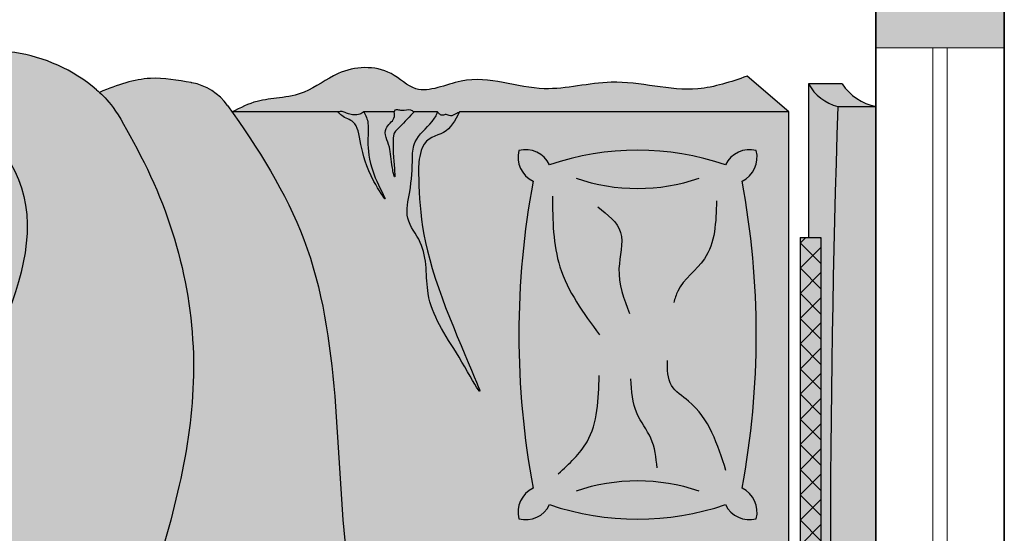
# Model space of a CAD drawing. Units: inches. Extents: x 3148 to 3962, y 1142 to 1671.
# Tile 5 of 9: x 3413 to 3482, y 1483 to 1519. Entities that reach past the tile are written whole.
import ezdxf

# ---------------------------------------------------------------- set-up
doc = ezdxf.new("R2010")
doc.units = ezdxf.units.IN
for name, color, linetype, lineweight in [('A-FURN', 8, 'Continuous', 18), ('A-GLAZ', 4, 'Continuous', 18), ('A-WALL', 7, 'Continuous', 35), ('estofado', 7, 'Continuous', 25)]:
    doc.layers.add(name, color=color, linetype=linetype, lineweight=lineweight)
doc.layers.add('A-WALL-PATT', color=252, linetype='Continuous', lineweight=13, true_color=0x939598)

# ---------------------------------------------------------------- blocks, each defined once
blk = doc.blocks.new('Cama Box Regencia LOLA')
at = {"layer": 'estofado', "ltscale": 0.2}
h = blk.add_hatch(color=256, dxfattribs=at)
h.dxf.hatch_style = 1
h.set_gradient(color1=(139, 102, 75), color2=(43, 31, 23), one_color=1, tint=0.1299999952316284)
h.paths.add_polyline_path([(-0.8097611300671587, -0.0676434826297623), (-0.8097611300671587, 0, -0.1973270565007711), (-0.8500000000000227, -0.060000000000116), (-0.8500000000000227, -0.1200000000000045, 0.2083477308151313)])
h = blk.add_hatch(color=256, dxfattribs=at)
h.dxf.hatch_style = 1
h.set_gradient(color1=(139, 102, 75), color2=(43, 31, 23), one_color=1, tint=0.1299999952316284, name='CURVED')
h.paths.add_polyline_path([(0.8097611300672723, 0), (-0.8097611300671587, 0), (-0.8097611300671587, -0.0676434826297054, 0.0166383680674931), (0.8097611300672723, -0.0676434823212162)])
h = blk.add_hatch(color=256, dxfattribs=at)
h.dxf.hatch_style = 1
h.set_gradient(color1=(139, 102, 75), color2=(43, 31, 23), one_color=1, tint=0.1299999952316284, name='INVCURVED')
h.paths.add_polyline_path([(0.8097611299908749, -0.0676434823237742, -0.0166383680667078), (-0.8097611300671587, -0.0676434826297623, -0.2083477308153697), (-0.8500000000001364, -0.1200000000000045), (-0.5763381074484643, -0.1200000000000045), (-0.5763381074485779, -0.0977075818103117), (0.5763381073808205, -0.0977075818103117), (0.5763381073808205, -0.1200000000000045), (0.8500000000000227, -0.1200000000000045, -0.2083477318100794)])
h = blk.add_hatch(color=256, dxfattribs=at)
h.dxf.hatch_style = 1
h.set_gradient(color1=(139, 102, 75), color2=(198, 169, 149), one_color=1, tint=0.6800000071525574, name='CYLINDER')
h.paths.add_polyline_path([(0.5763381073808205, -0.0977075818103686), (-0.5763381074484643, -0.0977075818103117), (-0.5763381074485779, -0.1348263709859339), (0.5763381073808205, -0.134826370985877)])
h = blk.add_hatch(dxfattribs=at)
h.set_pattern_fill('ANSI37,_O', color=256, scale=0.01)
h.set_pattern_definition([(45, (-24.74368160026529, -44.17612681992631), (-0.0224506403026729, 0.0224506403026729), []), (135, (-24.74368160026529, -44.17612681992631), (-0.0224506403026729, -0.0224506403026729), [])])
h.paths.add_polyline_path([(0.5763381073808205, -0.0977075818103686), (-0.5763381074484643, -0.0977075818103117), (-0.5763381074485779, -0.1348263709859339), (0.5763381073808205, -0.134826370985877)])
h = blk.add_hatch(color=256, dxfattribs=at)
h.dxf.hatch_style = 1
h.set_gradient(color1=(240, 232, 219), color2=(213, 190, 154), one_color=1, tint=0.7200000286102295)
edge = h.paths.add_edge_path()
edge.add_line((-0.8000000000000682, -0.1548023628405417), (-0.863597199697665, -0.2293271111754507))
edge.add_spline(control_points=[(-0.8635971996977787, -0.2293271111754507), (-0.8537222782123308, -0.258285373872468), (-0.8269013755602826, -0.3369378214810581), (-0.8674912876567759, -0.4595932758330151), (-0.8253488717912205, -0.6001498518888299), (-0.8771423076391329, -0.7139760714239288), (-0.8243323781925938, -0.8129899320257435), (-0.885044987287756, -0.8716602542656914), (-0.879518062107536, -0.9542863467743244), (-0.8339551707063037, -1.008464155856984), (-0.8245672924600739, -1.059984630119799), (-0.8208601923470268, -1.104655887174089), (-0.8073908324747662, -1.131238421004809), (-0.7999999999999546, -1.145824641594799)], knot_values=[0, 0, 0, 0, 0.0901802310564388, 0.2449351320798513, 0.3646438241986237, 0.5132330690395209, 0.5950634960661151, 0.646820388242338, 0.740988272125753, 0.8098674202588053, 0.8551784313864677, 0.8950360916221496, 0.9434986994854018, 0.9434986994854018, 0.9434986994854018, 0.9434986994854018], degree=3, periodic=0)
edge.add_line((-0.7999999999999546, -1.145824641594856), (-0.7999999999999546, -0.9571831923306604))
edge.add_spline(control_points=[(-0.8000000000001818, -0.9571831923294098), (-0.8003674620557603, -0.9560020588672273), (-0.8014778173377408, -0.9524330433489467), (-0.799534669348418, -0.9460450666617248), (-0.7963405736333016, -0.9382358308520792), (-0.7944188048602429, -0.9289040147384638), (-0.7953122817383474, -0.9190683391483389), (-0.7985341887020923, -0.9137677522519994), (-0.7999999999999546, -0.911356242470788)], knot_values=[0, 0, 0, 0, 0.0036609130031785, 0.0110621328900358, 0.0190316076023675, 0.0292873612819121, 0.0393286152452009, 0.0477100398955968, 0.0477100398955968, 0.0477100398955968, 0.0477100398955968], degree=3, periodic=0)
edge.add_line((-0.8000000000000682, -0.9113562424705037), (-0.7999999999999546, -0.8573491405791173))
edge.add_spline(control_points=[(-0.7999999999999546, -0.8573491405791173), (-0.8011509914009592, -0.8570771933481751), (-0.804102924754261, -0.8563797336621519), (-0.8039036519178353, -0.8498286502876908), (-0.8010279369466388, -0.8413595542568258), (-0.805623441450507, -0.8302818657685406), (-0.801318481758244, -0.8238273834048186), (-0.7999999999999546, -0.8218505664625013)], knot_values=[0, 0, 0, 0, 0.0032305881034183, 0.0082854491905874, 0.015951437769388, 0.0315866871777379, 0.0384893971878813, 0.0384893971878813, 0.0384893971878813, 0.0384893971878813], degree=3, periodic=0)
edge.add_line((-0.7999999999999546, -0.821850566462558), (-0.7999999999999546, -0.7800193173444541))
edge.add_spline(control_points=[(-0.7999999999999546, -0.7800193173443404), (-0.7985416092056994, -0.7788853679199974), (-0.7956241855360986, -0.7766169698310819), (-0.7929439183725436, -0.7707329795046576), (-0.7969680334608711, -0.7644035258254576), (-0.7912681985083055, -0.7566015403456845), (-0.7963938877088595, -0.7483952775559715), (-0.798936373489596, -0.7431699116222604), (-0.799999999999841, -0.7409839258539251)], knot_values=[0, 0, 0, 0, 0.0055481279082489, 0.0110986984731684, 0.0174746050947868, 0.0251556172852474, 0.035519246289823, 0.0429729849735991, 0.0429729849735991, 0.0429729849735991, 0.0429729849735991], degree=3, periodic=0)
edge.add_line((-0.7999999999999546, -0.740983925853584), (-0.8000000000000682, -0.1548023628405417))
h = blk.add_hatch(color=256, dxfattribs=at)
h.dxf.hatch_style = 1
h.set_gradient(color1=(240, 232, 219), color2=(213, 190, 154), one_color=1, tint=0.7200000286102295, name='CURVED')
edge = h.paths.add_edge_path()
edge.add_spline(control_points=[(0.343533776195045, -0.8455058148597345), (0.2879313990920309, -0.8167160606696484), (0.2054770794474052, -0.7744470032542381), (0.0954193394759386, -0.7742416952675626), (-0.0885363502328574, -0.7276964167006668), (0.2428192566063672, -0.7672518992321216), (0.345087521536243, -0.8076697826234067), (0.3825206986321063, -0.8228555492498799)], knot_values=[0.0056315103357428, 0.0056315103357428, 0.0056315103357428, 0.0056315103357428, 0.1860138916206105, 0.2660015162584448, 0.3570871810327863, 0.5963901805690979, 0.739731738908988, 0.739731738908988, 0.739731738908988, 0.739731738908988], degree=3, periodic=0)
edge.add_spline(control_points=[(0.3825206986325611, -0.8228555492497662), (0.3974221570828149, -0.8135511441712424), (0.4121061736600496, -0.8037181558521524), (0.4266849906532571, -0.7937075488799225)], knot_values=[1.358237767273279, 1.358237767273279, 1.358237767273279, 1.358237767273279, 1.409915662372559, 1.409915662372559, 1.409915662372559, 1.409915662372559], degree=3, periodic=0)
edge.add_spline(control_points=[(0.4266849905698109, -0.7937075489369932), (0.3998777739682282, -0.7821381809783361), (0.3476761897024971, -0.7634757898491671), (0.2670618099601825, -0.7565375622627358), (0.0835725072796549, -0.7192994417154637), (0.288524529784695, -0.7446405493717521), (0.4247448861246994, -0.7759943071475277), (0.4449816270193879, -0.7810438091316882)], knot_values=[0.1043639306803623, 0.1043639306803623, 0.1043639306803623, 0.1043639306803623, 0.1896363068641149, 0.2696239315019491, 0.3607095962762907, 0.6000125958126024, 0.6446217338078729, 0.6446217338078729, 0.6446217338078729, 0.6446217338078729], degree=3, periodic=0)
edge.add_spline(control_points=[(0.4449816270197289, -0.7810438091316882), (0.5029779388527232, -0.7406836481117695), (0.5966687145296419, -0.6736247633211292), (0.7071737530245628, -0.6656573253703187), (0.7517012483331201, -0.6672238302253392)], knot_values=[1.43159032281798, 1.43159032281798, 1.43159032281798, 1.43159032281798, 1.63814180148235, 1.770695287284994, 1.770695287284994, 1.770695287284994, 1.770695287284994], degree=3, periodic=0)
edge.add_arc((0.7481853615017826, -0.767162003811734), 0.0999999999999888, 58.7920033978138, 87.98512997550938, ccw=False)
edge.add_line((0.8000000000000682, -0.6816328085782289), (0.8000000000000682, -0.154802362840428))
edge.add_line((0.8000000000000682, -0.154802362840428), (-0.7999999999999546, -0.154802362840428))
edge.add_line((-0.7999999999999546, -0.154802362840428), (-0.8000000000000682, -0.7409839258539819))
edge.add_spline(control_points=[(-0.799999999999841, -0.7409839258539251), (-0.7846451382113174, -0.74846387981205), (-0.7568940913494089, -0.7651582159765554), (-0.7559936909002545, -0.8096905380045313), (-0.7049413305308008, -0.8142555457367848), (-0.7013836936888538, -0.8139988647640733)], knot_values=[0.0122267587020837, 0.0122267587020837, 0.0122267587020837, 0.0122267587020837, 0.0594720782072034, 0.1062176618094138, 0.134458043575382, 0.134458043575382, 0.134458043575382, 0.134458043575382], degree=3, periodic=0)
edge.add_spline(control_points=[(-0.7013836936890812, -0.8139988647637892), (-0.6428309483887916, -0.8132695376718857), (-0.532520673001045, -0.8118955240036598), (-0.2390712668254764, -0.6717984706609172), (-0.3892411364554391, -0.7557901092520752), (-0.4591093260188473, -0.8070101468627512), (-0.5571511178645779, -0.795652750469742), (-0.608497950975675, -0.8409486634728295), (-0.6632498050151981, -0.8266781836207997), (-0.6991149398675134, -0.8254126024436914), (-0.719552182989446, -0.8246914287938125)], knot_values=[0, 0, 0, 0, 0.2187005959148062, 0.4120203559900679, 0.4786136596093368, 0.6046444033330721, 0.6969970394608519, 0.7456449795902803, 0.7925683322559657, 0.8547274388453192, 0.8547274388453192, 0.8547274388453192, 0.8547274388453192], degree=3, periodic=0)
edge.add_spline(control_points=[(-0.7195521829781911, -0.824691428792164), (-0.7293124663336812, -0.8248308281530967), (-0.7545977292818407, -0.8216412233076653), (-0.7742556984202338, -0.794819860189591), (-0.7939222919129634, -0.7820064600295497), (-0.799999999999841, -0.7800193173443404)], knot_values=[0.1564883932805935, 0.1564883932805935, 0.1564883932805935, 0.1564883932805935, 0.184397548386913, 0.2313764834161266, 0.2505984550882281, 0.2505984550882281, 0.2505984550882281, 0.2505984550882281], degree=3, periodic=0)
edge.add_line((-0.8000000000000682, -0.7800193173444541), (-0.7999999999999546, -0.8218505664627286))
edge.add_spline(control_points=[(-0.7999999999999546, -0.8218505664625013), (-0.7938082505512511, -0.8290217081292894), (-0.7673857405620766, -0.8512914803976059), (-0.7619109683460011, -0.8661369353891359), (-0.6555700939965164, -0.8510070218793543), (-0.7139793977868294, -0.8637526923380391), (-0.7379026254519659, -0.8623504601624176), (-0.7688129786438367, -0.8813042143888196), (-0.7854260296310259, -0.8561610219318254), (-0.7961930533253962, -0.8566031243811949), (-0.7999999999999546, -0.8573491405791173)], knot_values=[0.0595743221876141, 0.0595743221876141, 0.0595743221876141, 0.0595743221876141, 0.08075289116965, 0.1037414994169835, 0.1697200936249022, 0.1760361327243865, 0.2071371586311508, 0.2404744334261798, 0.2623408547027293, 0.2736604507987723, 0.2736604507987723, 0.2736604507987723, 0.2736604507987723], degree=3, periodic=0)
edge.add_line((-0.7999999999999546, -0.8573491405791173), (-0.8000000000000682, -0.9113562424721521))
edge.add_spline(control_points=[(-0.8000000000000682, -0.9113562424720385), (-0.7937204054647964, -0.9077594990848183), (-0.7710343135782978, -0.8978798065321029), (-0.7213062468074442, -0.9144666877443228), (-0.6268586829058905, -0.862430497409548), (-0.6896594748232019, -0.9045634991654196), (-0.7483442493064559, -0.9189273406958591), (-0.7835301183422417, -0.922920432793262), (-0.7896301351460125, -0.9477657000142585), (-0.7975786973822779, -0.955260590410262), (-0.8000000000001818, -0.9571831923294098)], knot_values=[0.0138560263374175, 0.0138560263374175, 0.0138560263374175, 0.0138560263374175, 0.0348737775836104, 0.0888666909546002, 0.1078792274429341, 0.1267378491223226, 0.1587140219647659, 0.1937574699451985, 0.2174867851300671, 0.2267221218327879, 0.2267221218327879, 0.2267221218327879, 0.2267221218327879], degree=3, periodic=0)
edge.add_line((-0.7999999999999546, -0.957183192329296), (-0.7999999999999546, -1.145824641594742))
edge.add_spline(control_points=[(-0.8000000000002955, -1.145824641594913), (-0.7271039467997298, -1.094596787649038), (-0.4885706936571524, -0.9465888221489535), (-0.0701640902225336, -0.9707493165000187), (0.237911901821235, -0.902164522332157), (0.3435337762145991, -0.845505814843193)], knot_values=[0.1168958193629841, 0.1168958193629841, 0.1168958193629841, 0.1168958193629841, 0.3797203297758731, 0.9577018633805092, 1.31379338443587, 1.31379338443587, 1.31379338443587, 1.31379338443587], degree=3, periodic=0)
h.paths.add_polyline_path([(-0.6766340706021765, -0.6101327540145576, -0.3575266660906883), (-0.7312746368313583, -0.6354535276154252, -0.3575266660894137), (-0.7059538632299791, -0.5808129613865844, -0.1647847126465284), (-0.7059538632300928, -0.2676124402649407, -0.3575266660890756), (-0.7312746368312446, -0.2129718740360431, -0.3575266660908716), (-0.6766340706020629, -0.2382926476369676, -0.0925607043966334), (-0.1295169377724505, -0.2382926476369107, -0.3575266660898965), (-0.0748763715433825, -0.2129718740360431, -0.3575266660894428), (-0.1001971451446479, -0.2676124402649407, -0.1647847126465285), (-0.1001971451445343, -0.5808129613865844, -0.3575266660890756), (-0.0748763715433825, -0.6354535276154821, -0.3575266660898962), (-0.1295169377724505, -0.6101327540146145, -0.0925607043966531)], flags=16)
h.paths.add_polyline_path([(0.0748763715433825, -0.6354535276157094, -0.3575266660910266), (0.1001971451446479, -0.5808129613865844, -0.1647847126465284), (0.1001971451445343, -0.2676124402649407, -0.3575266660890757), (0.0748763715433825, -0.2129718740360431, -0.3575266660898962), (0.1295169377724505, -0.2382926476369107, -0.0925607043966334), (0.6766340706020629, -0.2382926476369676, -0.3575266660908718), (0.7312746368312446, -0.2129718740360431, -0.3575266660894425), (0.7059538632299791, -0.2676124402649407, -0.1647847126465283), (0.7059538632300928, -0.5808129613865844, -0.3575266660890756), (0.7312746368312446, -0.6354535276154821, -0.3575266660908716), (0.6766340706020629, -0.6101327540145576, -0.0925607043966335), (0.1295169377724505, -0.6101327540146145, -0.3575266660906303)], flags=16)
h = blk.add_hatch(color=256, dxfattribs=at)
h.dxf.hatch_style = 1
h.set_gradient(color1=(106, 82, 42), color2=(160, 123, 64), one_color=1, tint=0.4399999976158142, name='CURVED')
h.paths.add_polyline_path([(-0.1001971451445343, -0.2676124402650544, 0.3575266660914516), (-0.0748763715433825, -0.2129718740358157, 0.3575266660906303), (-0.1295169377724505, -0.2382926476369107, 0.0925607043966334), (-0.6766340706020629, -0.2382926476369676, 0.3575266660908717), (-0.7312746368312446, -0.2129718740360431, 0.3575266660886796), (-0.7059538632300928, -0.2676124402648838, 0.1647847126464969), (-0.7059538632300928, -0.5808129613864708, 0.3575266660910845), (-0.731274636831131, -0.6354535276157094, 0.3575266660898384), (-0.6766340706021765, -0.6101327540146145, 0.0925607043966531), (-0.1295169377724505, -0.6101327540146145, 0.3575266660898962), (-0.0748763715433825, -0.6354535276154821, 0.3575266660883126), (-0.1001971451444206, -0.5808129613866413, 0.164784712646497)])
h = blk.add_hatch(color=256, dxfattribs=at)
h.dxf.hatch_style = 1
h.set_gradient(color1=(206, 178, 131), color2=(227, 212, 186), one_color=1, tint=0.8100000023841857, name='CYLINDER')
edge = h.paths.add_edge_path()
edge.add_arc((0.7481853614966667, -0.7671620038115634), 0.0999999999999888, 342.0511336145294, 447.9851299725766)
edge.add_spline(control_points=[(0.7517012483331201, -0.6672238302253392), (0.7071737530245628, -0.6656573253703187), (0.5966687145298692, -0.6736247633211292), (0.5029779388527232, -0.7406836481117125), (0.4449816270195015, -0.7810438091316314)], knot_values=[1.431590322817835, 1.431590322817835, 1.431590322817835, 1.431590322817835, 1.564143808620479, 1.770695287284994, 1.770695287284994, 1.770695287284994, 1.770695287284994], degree=3, periodic=0)
edge.add_spline(control_points=[(0.4449816270195015, -0.7810438091316314), (0.4388957332065502, -0.7852790380018178), (0.4327996148541616, -0.7895089160493285), (0.4266849906533708, -0.7937075488798087)], knot_values=[1.409915662372814, 1.409915662372814, 1.409915662372814, 1.409915662372814, 1.431590322817835, 1.431590322817835, 1.431590322817835, 1.431590322817835], degree=3, periodic=0)
edge.add_spline(control_points=[(0.4266849906533708, -0.7937075488798087), (0.4121061736600496, -0.8037181558521524), (0.3974221570825875, -0.8135511441712991), (0.38252069863222, -0.8228555492498799)], knot_values=[1.358237767273037, 1.358237767273037, 1.358237767273037, 1.358237767273037, 1.409915662372815, 1.409915662372815, 1.409915662372815, 1.409915662372815], degree=3, periodic=0)
edge.add_line((0.3825206986330158, -0.8228555492493114), (0.343533776286904, -0.8455058148063584))
edge.add_spline(control_points=[(0.3435337761924302, -0.8455058148550165), (0.2379119018048641, -0.902164522335795), (-0.0701640902311738, -0.9707493164995071), (-0.4885706936571524, -0.9465888221488967), (-0.7271039467997298, -1.094596787649038), (-0.8000000000000682, -1.145824641594742)], knot_values=[0.1168958193630798, 0.1168958193630798, 0.1168958193630798, 0.1168958193630798, 0.472987340393773, 1.050968873998409, 1.313793384411202, 1.313793384411202, 1.313793384411202, 1.313793384411202], degree=3, periodic=0)
edge.add_spline(control_points=[(-0.8000000000000682, -1.145824641594742), (-0.8038896190357718, -1.14855807951244), (-0.8077744942224853, -1.151305646504738), (-0.8116551946761774, -1.154065647517199)], knot_values=[0.1028719158199011, 0.1028719158199011, 0.1028719158199011, 0.1028719158199011, 0.1168958193630799, 0.1168958193630799, 0.1168958193630799, 0.1168958193630799], degree=3, periodic=0)
edge.add_arc((-0.7536973518524519, -1.235557294053705), 0.1000000000000352, 125.4208969883762, 169.6981795679068)
edge.add_spline(control_points=[(-0.852085287466366, -1.217673946333093), (-0.8521399740518518, -1.217974812833915), (-0.8565649010855622, -1.242328483616745), (-0.8662697220019026, -1.297321141147904), (-0.8487158298532904, -1.34896742172242), (-0.8348745804664758, -1.381844109035796)], knot_values=[0.3128349436863077, 0.3128349436863077, 0.3128349436863077, 0.3128349436863077, 0.3137509534211996, 0.386958004641742, 0.4759027329026081, 0.4759027329026081, 0.4759027329026081, 0.4759027329026081], degree=3, periodic=0)
edge.add_spline(control_points=[(-0.8348745804664758, -1.38184410903591), (-0.8226532004149476, -1.367823298399059), (-0.8056354908857201, -1.352141651537124), (-0.7460155199962628, -1.32170802000337)], knot_values=[0.0062456970656236, 0.0062456970656236, 0.0062456970656236, 0.0062456970656236, 0.0554759259147193, 0.0554759259147193, 0.0554759259147193, 0.0554759259147193], degree=3, periodic=0)
edge.add_spline(control_points=[(-0.7460155200169539, -1.321708019985464), (-0.6188339616464873, -1.25080943574278), (-0.3488365122128698, -1.179158668568902), (0.0338148848931041, -1.279726484458706), (0.3977250465933366, -1.412092721352792), (0.6449024721503065, -1.106270719748692), (0.7873766543807506, -1.256744909425322), (0.8547271521993025, -1.327877176513538)], knot_values=[0.0991852523588446, 0.0991852523588446, 0.0991852523588446, 0.0991852523588446, 0.5236467270390676, 0.9270872950244264, 1.289918234564769, 1.564439021262726, 1.810554634340498, 1.810554634340498, 1.810554634340498, 1.810554634340498], degree=3, periodic=0)
edge.add_arc((0.5509678495186563, -1.223443291813453), 0.3212104454069235, 341.0267878798241, 383.7782184284114)
edge.add_arc((1.292676354991499, -0.9435407756057543), 0.4723459732861395, 162.0511336103901, 198.5657216587827, ccw=False)
h = blk.add_hatch(color=256, dxfattribs=at)
h.dxf.hatch_style = 1
h.set_gradient(color1=(240, 232, 219), color2=(137, 106, 57), one_color=1, tint=0.3799999952316284, name='CURVED')
edge = h.paths.add_edge_path()
edge.add_spline(control_points=[(-0.719552182989446, -0.8246914287938125), (-0.6991149398675134, -0.8254126024436914), (-0.6632498050151981, -0.8266781836207997), (-0.608497950975675, -0.8409486634728295), (-0.5571511178645779, -0.795652750469742), (-0.4591093260188473, -0.8070101468627512), (-0.3892411364554391, -0.7557901092520752), (-0.2390712668254764, -0.6717984706609172), (-0.532520673001045, -0.8118955240036598), (-0.6428309483887916, -0.8132695376718857), (-0.7013836936890812, -0.8139988647637892)], knot_values=[0, 0, 0, 0, 0.0621591065893537, 0.1090824592550391, 0.1577303993844675, 0.2500830355122473, 0.3761137792359825, 0.4427070828552515, 0.6360268429305131, 0.8547274388453192, 0.8547274388453192, 0.8547274388453192, 0.8547274388453192], degree=3, periodic=0)
edge.add_spline(control_points=[(-0.7013836936888538, -0.8139988647640733), (-0.7049413305308008, -0.8142555457367848), (-0.7559936909002545, -0.8096905380045313), (-0.7568940913494089, -0.7651582159765554), (-0.7846451382113174, -0.74846387981205), (-0.799999999999841, -0.7409839258539251)], knot_values=[0.0122267587020837, 0.0122267587020837, 0.0122267587020837, 0.0122267587020837, 0.0404671404680519, 0.0872127240702623, 0.134458043575382, 0.134458043575382, 0.134458043575382, 0.134458043575382], degree=3, periodic=0)
edge.add_spline(control_points=[(-0.799999999999841, -0.7409839258539251), (-0.798936373489596, -0.7431699116222604), (-0.7963938877088595, -0.7483952775559715), (-0.7912681985083055, -0.7566015403456845), (-0.7969680334608711, -0.7644035258254576), (-0.7929439183725436, -0.7707329795046576), (-0.7956241855360986, -0.7766169698310819), (-0.7985416092056994, -0.7788853679199974), (-0.7999999999999546, -0.7800193173443404)], knot_values=[0, 0, 0, 0, 0.0074537386837761, 0.0178173676883516, 0.0254983798788123, 0.0318742865004307, 0.0374248570653501, 0.0429729849735991, 0.0429729849735991, 0.0429729849735991, 0.0429729849735991], degree=3, periodic=0)
edge.add_spline(control_points=[(-0.799999999999841, -0.7800193173443404), (-0.7939222919129634, -0.7820064600295497), (-0.7742556984202338, -0.794819860189591), (-0.7545977292818407, -0.8216412233076653), (-0.7293124663336812, -0.8248308281530967), (-0.7195521829781911, -0.824691428792164)], knot_values=[0.1564883932805935, 0.1564883932805935, 0.1564883932805935, 0.1564883932805935, 0.175710364952695, 0.2226892999819086, 0.2505984550882281, 0.2505984550882281, 0.2505984550882281, 0.2505984550882281], degree=3, periodic=0)
h = blk.add_hatch(color=256, dxfattribs=at)
h.dxf.hatch_style = 1
h.set_gradient(color1=(240, 232, 219), color2=(137, 106, 57), one_color=1, tint=0.3799999952316284, name='CURVED')
edge = h.paths.add_edge_path()
edge.add_spline(control_points=[(0.3825206986321063, -0.8228555492498799), (0.345087521536243, -0.8076697826234067), (0.2428192566063672, -0.7672518992321216), (-0.0885363502328574, -0.7276964167006668), (0.0954193394759386, -0.7742416952675626), (0.2054770794474052, -0.7744470032542381), (0.2879313990920309, -0.8167160606696484), (0.343533776195045, -0.8455058148597345)], knot_values=[0.0056315103357428, 0.0056315103357428, 0.0056315103357428, 0.0056315103357428, 0.1489730686756328, 0.3882760682119444, 0.479361732986286, 0.5593493576241202, 0.739731738908988, 0.739731738908988, 0.739731738908988, 0.739731738908988], degree=3, periodic=0)
edge.add_line((0.343533776195045, -0.8455058148597913), (0.3825206986321063, -0.8228555492498799))
h = blk.add_hatch(color=256, dxfattribs=at)
h.dxf.hatch_style = 1
h.set_gradient(color1=(240, 232, 219), color2=(137, 106, 57), one_color=1, tint=0.3799999952316284, name='CURVED')
edge = h.paths.add_edge_path()
edge.add_spline(control_points=[(-0.7999999999999546, -0.8573491405791173), (-0.7961930533253962, -0.8566031243811949), (-0.7854260296310259, -0.8561610219318254), (-0.7688129786438367, -0.8813042143888196), (-0.7379026254519659, -0.8623504601624176), (-0.7139793977868294, -0.8637526923380391), (-0.6555700939965164, -0.8510070218793543), (-0.7619109683460011, -0.8661369353891359), (-0.7673857405620766, -0.8512914803976059), (-0.7938082505512511, -0.8290217081292894), (-0.7999999999999546, -0.8218505664625013)], knot_values=[0.0595743221876141, 0.0595743221876141, 0.0595743221876141, 0.0595743221876141, 0.0708939182836571, 0.0927603395602066, 0.1260976143552356, 0.1571986402619999, 0.1635146793614841, 0.2294932735694029, 0.2524818818167364, 0.2736604507987723, 0.2736604507987723, 0.2736604507987723, 0.2736604507987723], degree=3, periodic=0)
edge.add_spline(control_points=[(-0.7999999999999546, -0.8218505664625013), (-0.801318481758244, -0.8238273834048186), (-0.805623441450507, -0.8302818657685406), (-0.8010279369466388, -0.8413595542568258), (-0.8039036519178353, -0.8498286502876908), (-0.804102924754261, -0.8563797336621519), (-0.8011509914009592, -0.8570771933481751), (-0.7999999999999546, -0.8573491405791173)], knot_values=[0, 0, 0, 0, 0.0069027100101435, 0.0225379594184934, 0.030203947997294, 0.0352588090844631, 0.0384893971878813, 0.0384893971878813, 0.0384893971878813, 0.0384893971878813], degree=3, periodic=0)
h = blk.add_hatch(color=256, dxfattribs=at)
h.dxf.hatch_style = 1
h.set_gradient(color1=(240, 232, 219), color2=(137, 106, 57), one_color=1, tint=0.3799999952316284, name='CURVED')
edge = h.paths.add_edge_path()
edge.add_spline(control_points=[(-0.8000000000001818, -0.9571831923294098), (-0.7975786973822779, -0.955260590410262), (-0.7896301351460125, -0.9477657000142585), (-0.7835301183422417, -0.922920432793262), (-0.7483442493064559, -0.9189273406958591), (-0.6896594748232019, -0.9045634991654196), (-0.6268586829058905, -0.862430497409548), (-0.7213062468074442, -0.9144666877443228), (-0.7710343135782978, -0.8978798065321029), (-0.7937204054647964, -0.9077594990848183), (-0.8000000000000682, -0.9113562424720385)], knot_values=[0.0138560263374175, 0.0138560263374175, 0.0138560263374175, 0.0138560263374175, 0.0230913630401383, 0.0468206782250069, 0.0818641262054395, 0.1138402990478828, 0.1326989207272713, 0.1517114572156053, 0.205704370586595, 0.2267221218327879, 0.2267221218327879, 0.2267221218327879, 0.2267221218327879], degree=3, periodic=0)
edge.add_spline(control_points=[(-0.7999999999999546, -0.911356242470788), (-0.7985341887020923, -0.9137677522519994), (-0.7953122817383474, -0.9190683391483389), (-0.7944188048602429, -0.9289040147384638), (-0.7963405736333016, -0.9382358308520792), (-0.799534669348418, -0.9460450666617248), (-0.8014778173377408, -0.9524330433489467), (-0.8003674620557603, -0.9560020588672273), (-0.8000000000001818, -0.9571831923294098)], knot_values=[0, 0, 0, 0, 0.008381424650396, 0.0184226786136847, 0.0286784322932294, 0.0366479070055611, 0.0440491268924183, 0.0477100398955968, 0.0477100398955968, 0.0477100398955968, 0.0477100398955968], degree=3, periodic=0)
h = blk.add_hatch(color=256, dxfattribs=at)
h.dxf.hatch_style = 1
h.set_gradient(color1=(206, 178, 131), color2=(233, 221, 200), one_color=1, tint=0.8500000238418579, name='CURVED')
edge = h.paths.add_edge_path()
edge.add_spline(control_points=[(0.9233883396182136, -2.254908822900802), (0.9143712174658276, -2.237158585978875), (0.8971704820246486, -2.20329887728792), (0.9295105801843419, -2.140290914518345), (0.848651568119294, -2.10957861148239), (0.9047062348403186, -2.046222426005954), (0.8299480774321636, -1.990932361540615), (0.9387479200587449, -1.92692496801726), (0.8590435458045249, -1.86767849203585), (0.8322262745575699, -1.826028043643361), (0.8247981799574972, -1.810442049687992)], knot_values=[0, 0, 0, 0, 0.0575832900035364, 0.1098437972159638, 0.1698138218664432, 0.2255174829302509, 0.2824861515521905, 0.3632291183773252, 0.4509842065695901, 0.5012091817853866, 0.5012091817853866, 0.5012091817853866, 0.5012091817853866], degree=3, periodic=0)
edge.add_spline(control_points=[(0.8247981799572698, -1.810442049688447), (0.8512430237993839, -1.769990096378137), (0.8869160776755506, -1.705010622333873), (0.9070359522544322, -1.586338752195842), (0.8536462472426364, -1.488247672851343), (0.8944567470317679, -1.387739666353695), (0.8643796102055603, -1.342420998864781), (0.8547271521993025, -1.327877176513538)], knot_values=[0, 0, 0, 0, 0.1438744691785906, 0.2224893870322766, 0.3492927143212738, 0.4561786976395368, 0.5066917301592304, 0.5066917301592304, 0.5066917301592304, 0.5066917301592304], degree=3, periodic=0)
edge.add_spline(control_points=[(0.8547271521993025, -1.327877176513538), (0.7873766543807506, -1.256744909425322), (0.6449024721503065, -1.106270719748692), (0.3977250465933366, -1.412092721352792), (0.0338148848931041, -1.279726484458706), (-0.3488365122128698, -1.179158668568902), (-0.6188339616464873, -1.25080943574278), (-0.7460155200169539, -1.321708019985464)], knot_values=[0.0991852523588446, 0.0991852523588446, 0.0991852523588446, 0.0991852523588446, 0.3453008654366167, 0.6198216521345741, 0.9826525916749167, 1.386093159660275, 1.810554634340498, 1.810554634340498, 1.810554634340498, 1.810554634340498], degree=3, periodic=0)
edge.add_spline(control_points=[(-0.7460155199962628, -1.32170802000337), (-0.8056354908857201, -1.352141651537124), (-0.8226532004149476, -1.367823298399059), (-0.8348745804664758, -1.38184410903591)], knot_values=[0.0062456970656236, 0.0062456970656236, 0.0062456970656236, 0.0062456970656236, 0.0554759259147193, 0.0554759259147193, 0.0554759259147193, 0.0554759259147193], degree=3, periodic=0)
edge.add_spline(control_points=[(-0.8348745804664758, -1.38184410903591), (-0.8364250716851984, -1.383622888820184), (-0.8378983647115774, -1.385374937005849), (-0.8393716577378427, -1.387126985191514)], knot_values=[0, 0, 0, 0, 0.0062456970656236, 0.0062456970656236, 0.0062456970656236, 0.0062456970656236], degree=3, periodic=0)
edge.add_arc((-0.6180450437709624, -1.576392779500167), 0.2912164331649039, 139.4648411061637, 203.3711573294546)
edge.add_arc((-0.7011750866292914, -1.609837078845487), 0.2016528082906132, 204.0179006417974, 212.6189639884946)
edge.add_spline(control_points=[(-0.8710220093900034, -1.718537943240505), (-0.8696870122217887, -1.721658691442996), (-0.8597709916446092, -1.746046247230935), (-0.8464685798230674, -1.804421032451443), (-0.888988689927828, -1.889951451602371), (-0.8378676506146121, -1.973422824210047), (-0.8371590179440318, -2.05992368952792), (-0.8871569320951948, -2.144598622072578), (-0.908935644436724, -2.210906123939594), (-0.9233883398977695, -2.254908823284267)], knot_values=[0, 0, 0, 0, 0.0101500649009363, 0.0785829584511912, 0.1732273504791735, 0.2688802694005398, 0.3498050162211252, 0.4202002266429896, 0.5590752189863636, 0.5590752189863636, 0.5590752189863636, 0.5590752189863636], degree=3, periodic=0)
edge.add_ellipse((-0.9040800600764669, -2.258882422916315), major_axis=(0.0267880171833212, 0.0267880171833213), ratio=0.4535320972039226, start_angle=94.15910660291303, end_angle=123.37101895145429, ccw=False)
edge.add_ellipse((-0.8772920428931456, -2.232094405732993), major_axis=(0.0772920428927364, 0.0772920428927364), ratio=0.168252450050839, start_angle=-1.0527401173021644e-10, end_angle=156.3071135567154, ccw=False)
edge.add_line((-0.8000000000002955, -2.154802362840428), (0.7999592378284888, -2.154802362840428))
edge.add_arc((0.9462065466516378, -2.098298447668867), 0.1567831871334379, 200.9447658774159, 201.1244713640487, ccw=False)
edge.add_arc((1.115979327553759, -2.004946707326951), 0.3497136727815615, 205.2898146244752, 205.3730108333857)
edge.add_ellipse((0.8772920428930319, -2.232094405732993), major_axis=(-0.0772920428927364, 0.0772920428927364), ratio=0.168252450050839, start_angle=203.6928864432847, end_angle=359.99999999994674, ccw=False)
edge.add_ellipse((0.9040800600763532, -2.258882422916315), major_axis=(-0.0267880171833213, 0.0267880171833213), ratio=0.4535320972039226, start_angle=236.6289810485458, end_angle=265.84089339708703, ccw=False)
for p, q in [((-0.8097611300671587, -0.0676434826297054), (-0.8097611300671587, 0)), ((-0.5763381074485779, -0.0977075818103686), (0.5763381073808205, -0.0977075818103686)), ((-0.5763381074485779, -0.1348263709859339), (-0.5763381074485779, -0.0977075818103686)), ((-0.5763381074485779, -0.1348263709859339), (0.5763381073808205, -0.1348263709859339)), ((-0.7999999999999546, -0.154802362840428), (-0.8635971996977787, -0.2293271111754507))]:
    blk.add_line(p, q, dxfattribs=at)
for points in [[(0.8097611300672723, 0), (-0.8097611300671587, 0)], [(-0.8500000000000227, -0.060000000000116), (-0.8500000000000227, -0.1200000000000045), (-0.5763381074485779, -0.1200000000000045)], [(0.8000000000000682, -0.6816328085741361), (0.8000000000000682, -0.154802362840428), (-0.7999999999999546, -0.154802362840428), (-0.7999999999999546, -0.7409839258540956)], [(-0.7999999999999546, -0.7800193173443404), (-0.7999999999999546, -0.8218505664625013)], [(-0.7999999999999546, -0.8573491405790605), (-0.7999999999999546, -0.9113562424710153)], [(-0.7999999999999546, -0.9571831923292393), (-0.7999999999999546, -1.145824641594799)]]:
    blk.add_lwpolyline(points, dxfattribs=at)
for centre, radius, start, end in [((-0.9029365906352494, 0.0189948651997156), 0.0950919100450938, 303.8271063535092, 348.4775023778618), ((-0.8899769538815007, -0.0476343534641615), 0.0826737179530018, 298.9175773754458, 345.9938957157011), ((-4.6343303e-09, 24.25977121121599), 24.3408877974203, 268.0935593847751, 271.9064406368756), ((-0.6852907786285414, -0.2248498560688859), 0.047493175008304, 165.516646303857, 244.209945069049), ((-0.7193966547980608, -0.2589557322385758), 0.047493175008304, 25.79005493108792, 104.4833536962803), ((-0.4030755041873136, -1.703357436968531), 1.490385562932656, 79.42346065608027, 100.5765393439127), ((-0.0867543535765663, -0.2589557322385758), 0.047493175008304, 75.51664630371964, 154.2099450689121), ((-0.120860229745972, -0.2248498560688859), 0.047493175008304, 295.790054930951, 14.48335369614292), ((-0.243690300061985, -0.4242127008258194), 0.4880688921049917, 161.2852469077218, 198.7147530922607), ((-0.562460708312642, -0.4242127008258194), 0.4880688921049917, 341.2852469077393, 18.71475309227822), ((-1.002461858008359, -0.4242127008257626), 0.3387897965243698, 341.1598423418016, 18.84015765820971), ((0.19631084963396, -0.4242127008257626), 0.3387897965243698, 161.1598423417902, 198.8401576581983), ((-0.6852907786285414, -0.6235755455826393), 0.047493175008304, 115.790054930951, 194.4833536961429), ((-0.120860229745972, -0.6235755455826393), 0.047493175008304, 345.516646303857, 64.20994506904903), ((-0.7193966547980608, -0.5894696694129494), 0.047493175008304, 255.5166463037197, 334.2099450689121), ((-0.4030755041873136, 0.8549320353169491), 1.490385562932656, 259.4234606560872, 280.5765393439197), ((-0.0867543535765663, -0.5894696694129494), 0.047493175008304, 205.7900549310879, 284.4833536962804), ((-0.7536973518525656, -1.235557294053876), 0.1, 125.4208969883012, 169.6981794711674), ((-0.618045043771076, -1.576392779500224), 0.2912164331649248, 139.4648411061415, 203.3711573294531)]:
    blk.add_arc(centre, radius, start, end, dxfattribs=at)
for points, knots in [([(-0.8635971996977787, -0.2293271111754507), (-0.8537222782123597, -0.2582853738724713), (-0.8269013755602529, -0.3369378214810687), (-0.8674912876567628, -0.459593275832977), (-0.8253488717912105, -0.6001498518888299), (-0.8771423076387755, -0.7139760714238776), (-0.824332378192706, -0.8129899320257793), (-0.8850449872876955, -0.8716602542656513), (-0.8795180621076731, -0.9542863467744586), (-0.8339551707061605, -1.008464155856879), (-0.8245672924602526, -1.059984630119836), (-0.820860192346876, -1.104655887174075), (-0.8073908324747767, -1.131238421004865), (-0.7999999999999546, -1.145824641594799)], [0, 0, 0, 0, 0.0901802310564388, 0.2449351320798513, 0.3646438241986237, 0.5132330690395209, 0.5950634960661151, 0.646820388242338, 0.740988272125753, 0.8098674202588053, 0.8551784313864677, 0.8950360916221496, 0.9434986994854018, 0.9434986994854018, 0.9434986994854018, 0.9434986994854018]), ([(-0.1609929429250769, -0.2668120520876869), (-0.207361296664481, -0.2816189425177519), (-0.2673465842344797, -0.3007741531050562), (-0.3100088172549912, -0.3711986237053177), (-0.3410959220547441, -0.371113456673647), (-0.3573768361287648, -0.371068853062809)], [0, 0, 0, 0, 0.1404794637529129, 0.1817338842404631, 0.2270973195475621, 0.2270973195475621, 0.2270973195475621, 0.2270973195475621]), ([(-0.641547568925148, -0.2836087781224137), (-0.6039704843628328, -0.2846768301159754), (-0.539944686002343, -0.2864966328594507), (-0.4983244357833337, -0.3487001107148991), (-0.4673537235191868, -0.3577134183149331), (-0.460449429265168, -0.3597227530484019)], [0, 0, 0, 0, 0.1057518620258909, 0.1801855432155129, 0.2015394496060149, 0.2015394496060149, 0.2015394496060149, 0.2015394496060149]), ([(-0.1657269282603693, -0.3891622340328808), (-0.1839821155447316, -0.3912290170364152), (-0.2191851220416109, -0.3952145677934529), (-0.2641538569791404, -0.4324302667024541), (-0.3028411853428648, -0.4348886966416372), (-0.3243911361614664, -0.4362581125853354)], [0, 0, 0, 0, 0.0540396012867365, 0.1042090889319622, 0.1672963371706364, 0.1672963371706364, 0.1672963371706364, 0.1672963371706364]), ([(-0.630774277431101, -0.4946666993113809), (-0.6169895699779718, -0.4772535648042688), (-0.5885015945383536, -0.441266950663047), (-0.5131074616321869, -0.4662255111125919), (-0.4667910825139399, -0.4484404284426592), (-0.4408934738504513, -0.4384959742387196)], [0, 0, 0, 0, 0.0606588350328579, 0.1253597443752535, 0.2074214353097695, 0.2074214353097695, 0.2074214353097695, 0.2074214353097695]), ([(-0.6501439432536245, -0.5758072434303472), (-0.6067249420939599, -0.5753127958675333), (-0.5155219215609228, -0.5742741927209986), (-0.4416129136043037, -0.5203678897559305), (-0.402889750189047, -0.4921247481343585)], [0, 0, 0, 0, 0.1270530108164939, 0.2668789710677518, 0.2668789710677518, 0.2668789710677518, 0.2668789710677518]), ([(-0.1552772464440295, -0.5652394970176715), (-0.1730924483668451, -0.5457941389807961), (-0.2188221854511549, -0.4958799637506091), (-0.2880058022633399, -0.4937226941133118), (-0.3302371516485891, -0.4924058446629829)], [0, 0, 0, 0, 0.0765478869158952, 0.1964903209174588, 0.1964903209174588, 0.1964903209174588, 0.1964903209174588]), ([(-0.7013836936890812, -0.8139988647637892), (-0.6428309483887775, -0.8132695376718778), (-0.5325206730010296, -0.8118955240036225), (-0.2390712668254173, -0.6717984706608711), (-0.3892411364555083, -0.755790109252117), (-0.4591093260187714, -0.8070101468627889), (-0.5571511178644899, -0.795652750469717), (-0.6084979509757439, -0.8409486634728317), (-0.6632498050152652, -0.8266781836208043), (-0.6991149398675783, -0.8254126024437319), (-0.719552182989446, -0.8246914287938125)], [0, 0, 0, 0, 0.2187005959148062, 0.4120203559900679, 0.4786136596093368, 0.6046444033330721, 0.6969970394608519, 0.7456449795902803, 0.7925683322559657, 0.8547274388453192, 0.8547274388453192, 0.8547274388453192, 0.8547274388453192]), ([(-0.799999999999841, -0.7409839258539251), (-0.7989363734895372, -0.7431699116222815), (-0.7963938877087565, -0.7483952775559015), (-0.7912681985084682, -0.7566015403457877), (-0.796968033460866, -0.7644035258254169), (-0.7929439183725189, -0.7707329795046354), (-0.7956241855361271, -0.7766169698311071), (-0.7985416092057079, -0.7788853679200344), (-0.7999999999999546, -0.7800193173443404)], [0, 0, 0, 0, 0.0074537386837761, 0.0178173676883516, 0.0254983798788123, 0.0318742865004307, 0.0374248570653501, 0.0429729849735991, 0.0429729849735991, 0.0429729849735991, 0.0429729849735991]), ([(-0.799999999999841, -0.7409839258539251), (-0.7846451382113174, -0.74846387981205), (-0.7568940913494089, -0.7651582159765554), (-0.7559936909002545, -0.8096905380045313), (-0.7049413305308008, -0.8142555457367848), (-0.7013836936888538, -0.8139988647640733)], [0.0122267587020837, 0.0122267587020837, 0.0122267587020837, 0.0122267587020837, 0.0594720782072034, 0.1062176618094138, 0.134458043575382, 0.134458043575382, 0.134458043575382, 0.134458043575382]), ([(-0.7195521829781911, -0.824691428792164), (-0.7293124663336812, -0.8248308281530967), (-0.7545977292818407, -0.8216412233076653), (-0.7742556984202338, -0.794819860189591), (-0.7939222919129634, -0.7820064600295497), (-0.799999999999841, -0.7800193173443404)], [0.1564883932805935, 0.1564883932805935, 0.1564883932805935, 0.1564883932805935, 0.184397548386913, 0.2313764834161266, 0.2505984550882281, 0.2505984550882281, 0.2505984550882281, 0.2505984550882281]), ([(-0.7999999999999546, -0.8218505664625013), (-0.8013184817582112, -0.8238273834047737), (-0.8056234414505565, -0.8302818657685486), (-0.8010279369466333, -0.8413595542568746), (-0.8039036519179351, -0.8498286502876482), (-0.80410292475424, -0.8563797336621606), (-0.8011509914010776, -0.857077193348196), (-0.7999999999999546, -0.8573491405791173)], [0, 0, 0, 0, 0.0069027100101435, 0.0225379594184934, 0.030203947997294, 0.0352588090844631, 0.0384893971878813, 0.0384893971878813, 0.0384893971878813, 0.0384893971878813]), ([(-0.7999999999999546, -0.8218505664625013), (-0.7938082505512511, -0.8290217081292894), (-0.7673857405620766, -0.8512914803976059), (-0.7619109683460011, -0.8661369353891359), (-0.6555700939965164, -0.8510070218793543), (-0.7139793977868294, -0.8637526923380391), (-0.7379026254519659, -0.8623504601624176), (-0.7688129786438367, -0.8813042143888196), (-0.7854260296310259, -0.8561610219318254), (-0.7961930533253962, -0.8566031243811949), (-0.7999999999999546, -0.8573491405791173)], [0.0595743221876141, 0.0595743221876141, 0.0595743221876141, 0.0595743221876141, 0.08075289116965, 0.1037414994169835, 0.1697200936249022, 0.1760361327243865, 0.2071371586311508, 0.2404744334261798, 0.2623408547027293, 0.2736604507987723, 0.2736604507987723, 0.2736604507987723, 0.2736604507987723]), ([(-0.8116551946761774, -1.154065647517199), (-0.7350455857787211, -1.099579968801037), (-0.493473113061782, -0.9463057365681493), (-0.0701640902311738, -0.9707493164995071), (0.2379119018048641, -0.902164522335795), (0.3435337761924302, -0.8455058148550165)], [0.1028719158199011, 0.1028719158199011, 0.1028719158199011, 0.1028719158199011, 0.3797203297758731, 0.9577018633805092, 1.313793384411202, 1.313793384411202, 1.313793384411202, 1.313793384411202]), ([(-0.8000000000000682, -0.9113562424720385), (-0.7937204054647964, -0.9077594990848183), (-0.7710343135782978, -0.8978798065321029), (-0.7213062468074442, -0.9144666877443228), (-0.6268586829058905, -0.862430497409548), (-0.6896594748232019, -0.9045634991654196), (-0.7483442493064559, -0.9189273406958591), (-0.7835301183422417, -0.922920432793262), (-0.7896301351460125, -0.9477657000142585), (-0.7975786973822779, -0.955260590410262), (-0.8000000000001818, -0.9571831923294098)], [0.0138560263374175, 0.0138560263374175, 0.0138560263374175, 0.0138560263374175, 0.0348737775836104, 0.0888666909546002, 0.1078792274429341, 0.1267378491223226, 0.1587140219647659, 0.1937574699451985, 0.2174867851300671, 0.2267221218327879, 0.2267221218327879, 0.2267221218327879, 0.2267221218327879]), ([(-0.7999999999999546, -0.911356242470788), (-0.7985341887021342, -0.913767752252043), (-0.795312281738289, -0.9190683391482961), (-0.7944188048601522, -0.9289040147384582), (-0.7963405736334027, -0.9382358308520572), (-0.7995346693483358, -0.946045066661701), (-0.8014778173378848, -0.9524330433489994), (-0.800367462055735, -0.9560020588672482), (-0.8000000000001818, -0.9571831923294098)], [0, 0, 0, 0, 0.008381424650396, 0.0184226786136847, 0.0286784322932294, 0.0366479070055611, 0.0440491268924183, 0.0477100398955968, 0.0477100398955968, 0.0477100398955968, 0.0477100398955968]), ([(-0.7460155200169539, -1.321708019985464), (-0.6188339616464873, -1.25080943574278), (-0.3488365122128698, -1.179158668568902), (0.0338148848931041, -1.279726484458706), (0.3977250465933366, -1.412092721352792), (0.6449024721503065, -1.106270719748692), (0.7873766543807506, -1.256744909425322), (0.8547271521993025, -1.327877176513538)], [0.0991852523588446, 0.0991852523588446, 0.0991852523588446, 0.0991852523588446, 0.5236467270390676, 0.9270872950244264, 1.289918234564769, 1.564439021262726, 1.810554634340498, 1.810554634340498, 1.810554634340498, 1.810554634340498]), ([(-0.852085287466366, -1.217673946333093), (-0.8521399740518518, -1.217974812833915), (-0.8565649010855622, -1.242328483616745), (-0.8662697220019026, -1.297321141147904), (-0.8487158298532904, -1.34896742172242), (-0.8348745804664758, -1.381844109035796)], [0.3128349436863077, 0.3128349436863077, 0.3128349436863077, 0.3128349436863077, 0.3137509534211996, 0.386958004641742, 0.4759027329026081, 0.4759027329026081, 0.4759027329026081, 0.4759027329026081]), ([(-0.8337777191962914, -1.686127396833001), (-0.7936227331957753, -1.590003258421234), (-0.5563859991466416, -1.394748990587913), (-0.1321102153461879, -1.783182047565389), (0.1908245506583626, -1.429131816234075), (0.5373208507353411, -1.424480211867205), (0.720102724937533, -1.549855593291283), (0.836774155394778, -1.71068108627179)], [0.0299011711635954, 0.0299011711635954, 0.0299011711635954, 0.0299011711635954, 0.2769669118207226, 0.7971145189980146, 1.093669199334649, 1.464665995707328, 1.788488893467898, 1.788488893467898, 1.788488893467898, 1.788488893467898])]:
    blk.add_open_spline(points, degree=3, knots=knots, dxfattribs=at)
for points in [[(-0.8546555176860692, -1.326056226378227), (-0.8546255600027735, -1.326046411595029), (-0.8545956023194776, -1.326036596811775), (-0.8545656446361817, -1.326026782028861)], [(-0.8393716577378427, -1.387126985191514), (-0.8262854811396209, -1.371564831868056), (-0.8131993045412855, -1.356002678544541), (-0.7460155199962628, -1.32170802000337)]]:
    blk.add_open_spline(points, degree=3, dxfattribs=at)
blk = doc.blocks.new('WIN-72')
for p, q in [((0.0003062757873522, 72.00020003451709), (9.000306275787352, 72.00020003451709)), ((4.000306275787352, 72.00020003451687), (4.000306275788716, 0.0002000345168653)), ((5.000306275787352, 72.00020003451687), (5.000306275788716, 0.0002000345168653)), ((0.0003062757873522, 0.0002000345170927), (9.000306275787352, 0.0002000345170927))]:
    blk.add_line(p, q)

msp = doc.modelspace()

# ---------------------------------------------------------------- hatches: boundary and pattern name
at = {"layer": 'A-WALL-PATT'}
h = msp.add_hatch(color=256, dxfattribs=at)
h.dxf.hatch_style = 1
h.paths.add_polyline_path([(3203.042306275788, 1410.799200034518), (3194.042306275787, 1410.799200034518), (3194.042306275787, 1296.799200034517), (3203.042306275786, 1296.799200034517), (3203.042306275787, 1300.855382799943)])
h.paths.add_polyline_path([(3203.042306275778, 1281.799200034517), (3194.042306275787, 1281.799200034517), (3194.042306275787, 1212.799200034517), (3203.042306275788, 1212.799200034517)])
h.paths.add_polyline_path([(3326.042306275788, 1206.799200034517), (3203.042306275788, 1206.799200034517), (3203.042306275788, 1197.799200034517), (3326.042306275788, 1197.799200034517)])
h.paths.add_polyline_path([(3341.042306275787, 1362.799200034517), (3335.042306275788, 1362.799200034517), (3335.042306275788, 1290.799200034517), (3341.042306275787, 1290.799200034517)])
h.paths.add_polyline_path([(3341.042306275788, 1207.799200034517), (3335.042306275788, 1207.799200034517), (3335.042306275788, 1206.799200034517), (3341.042306275788, 1206.799200034517)])
h.paths.add_polyline_path([(3341.042306275787, 1259.799200034517), (3335.042306275788, 1259.799200034517), (3335.042306275788, 1255.799200034517), (3341.042306275787, 1255.799200034517)])
h.paths.add_polyline_path([(3341.042306275787, 1281.799200034517), (3335.042306275788, 1281.799200034517), (3335.042306275788, 1277.799200034517), (3341.042306275787, 1277.799200034517)])
h.paths.add_polyline_path([(3377.042306275787, 1287.799200034517), (3350.042306275788, 1287.799200034517), (3350.042306275788, 1281.799200034517), (3377.042306275787, 1281.799200034517)])
h.paths.add_polyline_path([(3473.042306275787, 1287.799200034517), (3445.042307275787, 1287.799200034517), (3437.042306275787, 1287.799200034517), (3437.042306275788, 1281.799200034517), (3473.042306275787, 1281.799200034517)])
h.paths.add_polyline_path([(3482.042306275788, 1313.299200034517), (3473.042306275787, 1313.299200034517), (3473.042306275787, 1296.799200034517), (3482.042306275788, 1296.799200034517)])
h.paths.add_polyline_path([(3482.042306275788, 1410.799200034517), (3473.042306275787, 1410.799200034517), (3473.042306275787, 1385.299200034517), (3482.042306275788, 1385.299200034517)])
h.paths.add_polyline_path([(3473.042306275787, 1416.799200034517), (3344.042306275788, 1416.799200034517), (3344.042306275788, 1410.799200034517), (3473.042306275787, 1410.799200034517)])
h.paths.add_polyline_path([(3482.042306275788, 1445.299200034517), (3473.042306275787, 1445.299200034517), (3473.042306275787, 1425.799200034517), (3482.042306275788, 1425.799200034517)])
h.paths.add_polyline_path([(3341.042306275787, 1426.299200034517), (3335.042306275788, 1426.299200034517), (3335.042306275788, 1425.799200034517), (3341.042306275787, 1425.799200034517)])
h.paths.add_polyline_path([(3304.042306275788, 1428.799200034517), (3253.542306275787, 1428.799200034517), (3253.542306275788, 1430.299200034517), (3251.042306275788, 1430.299200034517), (3251.042306275787, 1428.799200034517), (3203.042306275788, 1428.799200034517), (3203.042306275788, 1512.799200034517), (3215.042306275788, 1512.799200034517), (3215.042306275788, 1518.799200034517), (3203.042306275788, 1518.799200034517), (3203.042306275788, 1539.799200034517), (3194.042306275787, 1539.799200034517), (3194.042306275787, 1425.799200034519), (3203.042306275787, 1425.799200034519), (3203.042306275787, 1422.799200034517), (3304.042306275788, 1422.799200034517)])
h.paths.add_polyline_path([(3265.542306275789, 1518.799200034517), (3239.042306275788, 1518.799200034517), (3239.042306275788, 1512.799200034517), (3251.042306275788, 1512.799200034517), (3251.042306275788, 1461.299200034517), (3253.542306275789, 1461.299200034517), (3253.542306275789, 1462.299200034517), (3255.542306275788, 1462.299200034517), (3255.542306275788, 1464.799200034517), (3253.542306275789, 1464.799200034517), (3253.542306275788, 1512.799200034517), (3265.542306275789, 1512.799200034517)], flags=17)
h.paths.add_polyline_path([(3307.542306275788, 1518.799200034517), (3289.542306275789, 1518.799200034517), (3289.542306275789, 1512.799200034517), (3301.542306275788, 1512.799200034517), (3301.542306275788, 1464.799200034517), (3286.542306275788, 1464.799200034517), (3286.542306275788, 1462.299200034517), (3304.042306275788, 1462.299200034517), (3304.042306275788, 1512.799200034517), (3307.542306275788, 1512.799200034517)])
h.paths.add_polyline_path([(3341.042306275787, 1539.799200034517), (3335.042306275788, 1539.799200034517), (3335.042306275788, 1518.799200034517), (3331.542306275788, 1518.799200034517), (3331.542306275788, 1512.799200034517), (3335.042306275788, 1512.799200034517), (3335.042306275788, 1462.299200034517), (3341.042306275787, 1462.299200034517)])
h.paths.add_polyline_path([(3335.042306275788, 1554.799200034517), (3203.042306275788, 1554.799200034517), (3203.042306275788, 1545.799200034517), (3335.042306275788, 1545.799200034517)])
h.paths.add_polyline_path([(3473.042306275787, 1554.799200034517), (3344.042306275787, 1554.799200034517), (3344.042306275787, 1545.799200034517), (3362.939954275788, 1545.799200034517), (3473.042306275787, 1545.799200034517)])
h.paths.add_polyline_path([(3482.042306275788, 1539.799200034517), (3473.042306275787, 1539.799200034517), (3473.042306275787, 1517.299200034517), (3482.042306275788, 1517.299200034517)])

# ---------------------------------------------------------------- linework, layer by layer
at = {"layer": 'A-WALL'}
for p, q in [((3482.042306275788, 1554.799200034517), (3482.042306275788, 1281.799200034517)), ((3473.042306275787, 1545.799200034517), (3473.042306275787, 1416.799200034517))]:
    msp.add_line(p, q, dxfattribs=at)

# ---------------------------------------------------------------- block references
at = {"layer": 'A-FURN', "xscale": 39.3701, "yscale": 39.3701, "zscale": 39.3701, "rotation": 270}
msp.add_blockref('Cama Box Regencia LOLA', (3473.042306275787, 1481.299200034517), dxfattribs=at)
at = {"layer": 'A-GLAZ'}
msp.add_blockref('WIN-72', (3473.042, 1445.299), dxfattribs=at)

doc.saveas('drawing.dxf')
